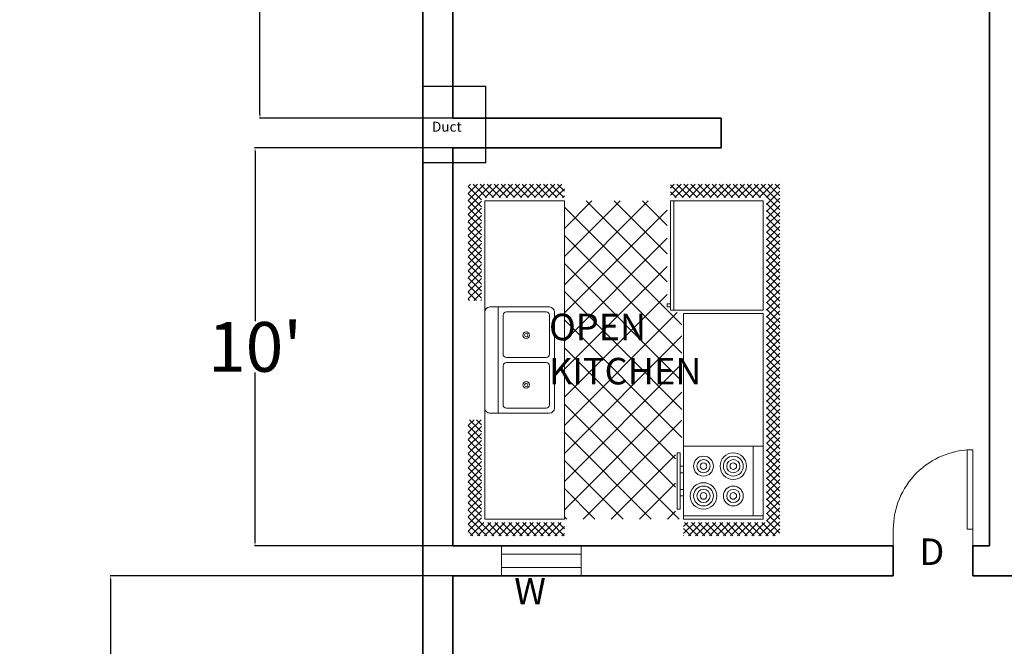
# Model space of a CAD drawing. Units: inches. Extents: x 371 to 1095, y -45 to 1219.
# Tile 8 of 18: x 371 to 668, y 421 to 610. Entities that reach past the tile are written whole.
import ezdxf

# ---------------------------------------------------------------- set-up
doc = ezdxf.new("R2010")
doc.units = ezdxf.units.IN
doc.header["$MEASUREMENT"] = 0
for name, color, linetype, lineweight in [('A-ANNO-DIMS', 2, 'Continuous', 18), ('A-ANNO-TEXT', 7, 'Continuous', 18), ('A-AREA-IDEN', 7, 'Continuous', 18), ('A-DOOR', 3, 'Continuous', 18), ('A-FLOR-FIXT', 9, 'Continuous', 18), ('A-FLOR-SHFT', 7, 'Continuous', 25), ('A-GLAZ', 4, 'Continuous', 18), ('A-WALL', 40, 'Continuous', 35), ('C-SITE-WALL', 40, 'Continuous', 35)]:
    doc.layers.add(name, color=color, linetype=linetype, lineweight=lineweight)
doc.styles.get("Standard").update_dxf_attribs({"font": 'arial.ttf'})
doc.dimstyles.get("Standard").update_dxf_attribs({"dimtxt": 1, "dimasz": 1, "dimexe": 0.18, "dimexo": 0.0625, "dimgap": 0.09, "dimtad": 0, "dimtih": 1, "dimtoh": 1, "dimdec": 0, "dimzin": 0, "dimdsep": 46, "dimlunit": 3, "dimtxsty": 'Standard', "dimcen": 0.09, "dimadec": 0, "dimazin": 0, "dimtfac": 1, "dimtdec": 0, "dimtofl": 0, "dimtmove": 0, "dimatfit": 3, "dimfxl": 1, "dimtolj": 1, "dimtzin": 0, "dimarcsym": 0})

# ---------------------------------------------------------------- blocks, each defined once
blk = doc.blocks.new('*U12')
for p, q in [((0, 0), (0, 5)), ((24, 0), (24, 5))]:
    blk.add_line(p, q)
blk.add_lwpolyline([(0, 0), (0, -24), (1.75, -24), (1.75, 0)], close=True)
blk.add_arc((0, 0), 24, 270, 0)
blk = doc.blocks.new('Kitchen Layout - 7 x 8 ft')
for p, q in [((-5, 81.32), (2.68, 89)), ((-5, 83.44), (0.56, 89)), ((-5, 85.56), (-1.56, 89)), ((-5, 87.68), (-3.68, 89)), ((-1, 84.97), (-5, 88.97)), ((-1, 82.85), (-5, 86.85)), ((1.09, 85), (-2.91, 89)), ((3.21, 85), (-0.79, 89)), ((0.81, 85), (4.81, 89)), ((5.34, 85), (1.34, 89)), ((2.93, 85), (6.93, 89)), ((7.46, 85), (3.46, 89)), ((5.05, 85), (9.05, 89)), ((9.58, 85), (5.58, 89)), ((7.17, 85), (11.17, 89)), ((11.7, 85), (7.7, 89)), ((9.29, 85), (13.29, 89)), ((13.82, 85), (9.82, 89)), ((11.41, 85), (15.41, 89)), ((15.94, 85), (11.94, 89)), ((13.53, 85), (17.53, 89)), ((18.06, 85), (14.06, 89)), ((15.65, 85), (19.65, 89)), ((20.18, 85), (16.18, 89)), ((17.78, 85), (21.78, 89)), ((22.31, 85), (18.31, 89)), ((19.9, 85), (23.9, 89)), ((24.43, 85), (20.43, 89)), ((22.02, 85), (26.02, 89)), ((26.55, 85), (22.55, 89)), ((24.14, 85), (28.14, 89)), ((28.67, 85), (24.67, 89)), ((26.26, 85), (30.26, 89)), ((30.79, 85), (26.79, 89)), ((28.38, 85), (32.38, 89)), ((32.91, 85), (28.91, 89)), ((30.5, 85), (34.5, 89)), ((35.03, 85), (31.03, 89)), ((32.63, 85), (36.63, 89)), ((37.16, 85), (33.16, 89)), ((34.75, 85), (38.75, 89)), ((39.28, 85), (35.28, 89)), ((36.87, 85), (40.87, 89)), ((41.4, 85), (37.4, 89)), ((38.99, 85), (42.99, 89)), ((43.52, 85), (39.52, 89)), ((41.11, 85), (45.11, 89)), ((45.64, 85), (41.64, 89)), ((43.23, 85), (47.23, 89)), ((47.76, 85), (43.76, 89)), ((45.35, 85), (49.35, 89)), ((49.88, 85), (45.88, 89)), ((47.47, 85), (51.47, 89)), ((52, 85), (48, 89)), ((49.6, 85), (53.6, 89)), ((54.13, 85), (50.13, 89)), ((51.72, 85), (55.72, 89)), ((56.25, 85), (52.25, 89)), ((53.84, 85), (57.84, 89)), ((58.37, 85), (54.37, 89)), ((55.96, 85), (59.96, 89)), ((60.49, 85), (56.49, 89)), ((58.08, 85), (62.08, 89)), ((62.61, 85), (58.61, 89)), ((60.2, 85), (64.2, 89)), ((64.73, 85), (60.73, 89)), ((62.32, 85), (66.32, 89)), ((66.85, 85), (62.85, 89)), ((64.45, 85), (68.45, 89)), ((68.97, 85), (64.97, 89)), ((66.57, 85), (70.57, 89)), ((71.1, 85), (67.1, 89)), ((68.69, 85), (72.69, 89)), ((73.22, 85), (69.22, 89)), ((70.81, 85), (74.81, 89)), ((75.34, 85), (71.34, 89)), ((72.93, 85), (76.93, 89)), ((77.46, 85), (73.46, 89)), ((75.05, 85), (79.05, 89)), ((79.58, 85), (75.58, 89)), ((77.17, 85), (81.17, 89)), ((81.7, 85), (77.7, 89)), ((79.29, 85), (83.29, 89)), ((83.82, 85), (79.82, 89)), ((81.42, 85), (85.42, 89)), ((85.95, 85), (81.95, 89)), ((83.54, 85), (87.54, 89)), ((88.07, 85), (84.07, 89)), ((85.66, 85), (89.66, 89)), ((90.19, 85), (86.19, 89)), ((87.78, 85), (91.78, 89)), ((92.31, 85), (88.31, 89)), ((89.9, 85), (93.9, 89)), ((94.43, 85), (90.43, 89)), ((92.02, 85), (96.02, 89)), ((96.55, 85), (92.55, 89)), ((94.14, 85), (98.14, 89)), ((101, 82.67), (94.67, 89)), ((96.27, 85), (100.27, 89)), ((101, 84.79), (96.79, 89)), ((97, 83.61), (101, 87.61)), ((101, 86.92), (98.92, 89)), ((-1, 80.73), (-5, 84.73)), ((34, 84), (96, 84)), ((34, 60), (34, 84)), ((96, 84), (96, 60)), ((97, 81.49), (101, 85.49)), ((101, 80.55), (97, 84.55)), ((97, 79.37), (101, 83.37)), ((-5, 79.19), (-1, 83.19)), ((-1, 78.61), (-5, 82.61)), ((-5, 77.07), (-1, 81.07)), ((-1, 76.49), (-5, 80.49)), ((74, 81), (95, 81)), ((101, 78.43), (97, 82.43)), ((97, 77.25), (101, 81.25)), ((101, 76.31), (97, 80.31)), ((-5, 74.95), (-1, 78.95)), ((-1, 74.36), (-5, 78.36)), ((97, 75.13), (101, 79.13)), ((101, 74.19), (97, 78.19)), ((-5, 72.83), (-1, 76.83)), ((-1, 72.24), (-5, 76.24)), ((-5, 70.71), (-1, 74.71)), ((97, 73.01), (101, 77.01)), ((101, 72.07), (97, 76.07)), ((97, 70.89), (101, 74.89)), ((-1, 70.12), (-5, 74.12)), ((-5, 68.59), (-1, 72.59)), ((-1, 68), (-5, 72)), ((101, 69.95), (97, 73.95)), ((97, 68.76), (101, 72.76)), ((101, 67.82), (97, 71.82)), ((-5, 66.47), (-1, 70.47)), ((-1, 65.88), (-5, 69.88)), ((97, 66.64), (101, 70.64)), ((101, 65.7), (97, 69.7)), ((97, 64.52), (101, 68.52)), ((-5, 64.35), (-1, 68.35)), ((-1, 63.76), (-5, 67.76)), ((-5, 62.22), (-1, 66.22)), ((-1, 61.64), (-5, 65.64)), ((101, 63.58), (97, 67.58)), ((97, 62.4), (101, 66.4)), ((101, 61.46), (97, 65.46)), ((-5, 60.1), (-1, 64.1)), ((-1, 59.52), (-5, 63.52)), ((97, 60.28), (101, 64.28)), ((100.34, 60), (97, 63.34)), ((-5, 57.98), (-1, 61.98)), ((-1, 57.39), (-5, 61.39)), ((-4.86, 56), (-1, 59.86)), ((10.4, 24), (45.9, 59.5)), ((18.88, 24), (54.38, 59.5)), ((27.37, 24), (62.87, 59.5)), ((33.03, 55.11), (37.41, 59.5)), ((96, 60), (34, 60)), ((35.85, 24), (71.35, 59.5)), ((76.2, 24), (40.7, 59.5)), ((84.68, 24), (49.18, 59.5)), ((93.17, 24), (57.67, 59.5)), ((96, 29.65), (66.15, 59.5)), ((80, 60), (80, 59)), ((82, 59), (82, 60)), ((87, 59), (87, 60)), ((89, 60), (89, 59)), ((98.22, 60), (97, 61.22)), ((98.84, 60), (101, 62.16)), ((100.96, 60), (101, 60.04)), ((-1.73, 56), (-5, 59.27)), ((-3.85, 56), (-5, 57.15)), ((-2.74, 56), (-1, 57.74)), ((0, 57), (33, 57)), ((67.71, 24), (33.68, 58.04)), ((44.34, 24), (77.84, 57.5)), ((52.82, 24), (86.32, 57.5)), ((61.31, 24), (96, 58.69)), ((96, 38.14), (76.64, 57.5)), ((96, 46.63), (85.13, 57.5)), ((96, 55.11), (93.57, 57.54)), ((0, 30.57), (24.43, 55)), ((0, 39.06), (15.94, 55)), ((0, 47.54), (7.46, 55)), ((1.91, 24), (32.91, 55)), ((33.77, 24), (2.77, 55)), ((42.26, 24), (11.26, 55)), ((50.74, 24), (19.74, 55)), ((59.23, 24), (28.23, 55)), ((31, 55), (31, 56)), ((32, 55), (31, 55)), ((32, 56), (32, 55)), ((25.29, 24), (0, 49.29)), ((69.79, 24), (96, 50.21)), ((78.28, 24), (96, 41.72)), ((16.8, 24), (0, 40.8)), ((86.76, 24), (96, 33.24)), ((8.32, 24), (0, 32.32)), ((-5, 21.92), (-2.92, 24)), ((-5, 19.8), (-1, 23.8)), ((-1, 21.33), (-3.67, 24)), ((-1, 23.45), (-1.55, 24)), ((0, 24), (96, 24)), ((0, 0), (0, 24)), ((95.25, 24), (96, 24.75)), ((96, 24), (96, 0)), ((97, 22.1), (98.9, 24)), ((97, 19.97), (101, 23.97)), ((101, 21.16), (98.16, 24)), ((101, 23.28), (100.28, 24)), ((-1, 19.21), (-5, 23.21)), ((-5, 17.68), (-1, 21.68)), ((-1, 17.09), (-5, 21.09)), ((101, 19.03), (97, 23.03)), ((97, 17.85), (101, 21.85)), ((101, 16.91), (97, 20.91)), ((-5, 15.55), (-1, 19.55)), ((-1, 14.97), (-5, 18.97)), ((47.25, 6.5), (47.25, 18.5)), ((48.75, 18.5), (48.75, 6.5)), ((97, 15.73), (101, 19.73)), ((101, 14.79), (97, 18.79)), ((-5, 13.43), (-1, 17.43)), ((-1, 12.85), (-5, 16.85)), ((-5, 11.31), (-1, 15.31)), ((97, 13.61), (101, 17.61)), ((101, 12.67), (97, 16.67)), ((97, 11.49), (101, 15.49)), ((-1, 10.73), (-5, 14.73)), ((-5, 9.19), (-1, 13.19)), ((-1, 8.6), (-5, 12.6)), ((101, 10.55), (97, 14.55)), ((97, 9.37), (101, 13.37)), ((101, 8.43), (97, 12.43)), ((-5, 7.07), (-1, 11.07)), ((-1, 6.48), (-5, 10.48)), ((-5, 4.95), (-1, 8.95)), ((97, 7.25), (101, 11.25)), ((101, 6.31), (97, 10.31)), ((97, 5.12), (101, 9.12)), ((-1, 4.36), (-5, 8.36)), ((-5, 2.83), (-1, 6.83)), ((-1, 2.24), (-5, 6.24)), ((101, 4.18), (97, 8.18)), ((97, 3), (101, 7)), ((101, 2.06), (97, 6.06)), ((-5, 0.71), (-1, 4.71)), ((-1, 0.12), (-5, 4.12)), ((64, 4), (32, 4)), ((97, 0.88), (101, 4.88)), ((101, -0.06), (97, 3.94)), ((-5, -1.42), (-1, 2.58)), ((2, -5), (-5, 2)), ((-5, -3.54), (-1, 0.46)), ((96, 0), (0, 0)), ((93.24, -5), (101, 2.76)), ((95.36, -5), (101, 0.64)), ((101, -2.18), (97, 1.82)), ((-0.12, -5), (-5, -0.12)), ((-2.25, -5), (-5, -2.25)), ((-4.34, -5), (-0.34, -1)), ((-2.22, -5), (1.78, -1)), ((-0.1, -5), (3.9, -1)), ((4.12, -5), (0.12, -1)), ((2.02, -5), (6.02, -1)), ((6.24, -5), (2.24, -1)), ((4.14, -5), (8.14, -1)), ((8.36, -5), (4.36, -1)), ((6.27, -5), (10.27, -1)), ((10.48, -5), (6.48, -1)), ((8.39, -5), (12.39, -1)), ((12.6, -5), (8.6, -1)), ((10.51, -5), (14.51, -1)), ((14.73, -5), (10.73, -1)), ((12.63, -5), (16.63, -1)), ((16.85, -5), (12.85, -1)), ((14.75, -5), (18.75, -1)), ((18.97, -5), (14.97, -1)), ((16.87, -5), (20.87, -1)), ((21.09, -5), (17.09, -1)), ((18.99, -5), (22.99, -1)), ((23.21, -5), (19.21, -1)), ((21.11, -5), (25.11, -1)), ((25.33, -5), (21.33, -1)), ((23.24, -5), (27.24, -1)), ((27.45, -5), (23.45, -1)), ((25.36, -5), (29.36, -1)), ((29.57, -5), (25.57, -1)), ((27.48, -5), (30, -2.48)), ((30, -3.3), (27.7, -1)), ((30, -1.18), (29.82, -1)), ((66, -2.54), (67.54, -1)), ((66, -4.66), (69.66, -1)), ((69.88, -5), (66, -1.12)), ((67.78, -5), (71.78, -1)), ((72, -5), (68, -1)), ((69.9, -5), (73.9, -1)), ((74.12, -5), (70.12, -1)), ((72.03, -5), (76.03, -1)), ((76.24, -5), (72.24, -1)), ((74.15, -5), (78.15, -1)), ((78.36, -5), (74.36, -1)), ((76.27, -5), (80.27, -1)), ((80.49, -5), (76.49, -1)), ((78.39, -5), (82.39, -1)), ((82.61, -5), (78.61, -1)), ((80.51, -5), (84.51, -1)), ((84.73, -5), (80.73, -1)), ((82.63, -5), (86.63, -1)), ((86.85, -5), (82.85, -1)), ((84.75, -5), (88.75, -1)), ((88.97, -5), (84.97, -1)), ((86.88, -5), (90.88, -1)), ((91.09, -5), (87.09, -1)), ((89, -5), (93, -1)), ((93.21, -5), (89.21, -1)), ((91.12, -5), (95.12, -1)), ((95.34, -5), (91.34, -1)), ((97.46, -5), (93.46, -1)), ((99.58, -5), (95.58, -1)), ((101, -4.3), (97, -0.3)), ((97.48, -5), (101, -1.48)), ((-4.37, -5), (-5, -4.37)), ((29.6, -5), (30, -4.6)), ((67.76, -5), (66, -3.24)), ((99.6, -5), (101, -3.6))]:
    blk.add_line(p, q)
for points in [[(0, 56), (0, 84), (33, 84), (33, 56)], [(74, 60), (74, 84), (95, 84), (95, 60)], [(76, 58), (76, 59), (93, 59), (93, 58)]]:
    blk.add_lwpolyline(points, close=True)
for points in [[(33.5, 21), (62.5, 21)], [(32, 1.5), (32, 19.5)], [(33.5, 6.5), (33.5, 18.5)], [(34.5, 19.5), (46.25, 19.5)], [(49.75, 19.5), (61.5, 19.5)], [(62.5, 18.5), (62.5, 6.5)], [(64, 19.5), (64, 1.5)], [(46.25, 5.5), (34.5, 5.5)], [(61.5, 5.5), (49.75, 5.5)], [(62.5, 0), (33.5, 0)]]:
    blk.add_lwpolyline(points)
for centre, radius in [((80, 75), 4), ((80, 75), 3), ((89, 75), 3), ((80, 75), 2), ((80, 75), 1), ((89, 75), 2), ((89, 75), 1), ((80, 66), 3), ((89, 66), 4), ((89, 66), 3), ((80, 66), 2), ((80, 66), 1), ((89, 66), 2), ((89, 66), 1), ((40.5, 12.5), 1), ((40.5, 12.5), 0.5), ((55.5, 12.5), 1), ((55.5, 12.5), 0.5)]:
    blk.add_circle(centre, radius)
for centre, radius, start, end in [((33.5, 19.5), 1.5, 90, 180), ((62.5, 19.5), 1.5, 0, 90), ((34.5, 18.5), 1, 90, 180), ((46.25, 18.5), 1, 0, 90), ((49.75, 18.5), 1, 90, 180), ((61.5, 18.5), 1, 0, 90), ((34.5, 6.5), 1, 180, 270), ((46.25, 6.5), 1, 270, 0), ((49.75, 6.5), 1, 180, 270), ((61.5, 6.5), 1, 270, 0), ((33.5, 1.5), 1.5, 180, 270), ((62.5, 1.5), 1.5, 270, 0)]:
    blk.add_arc(centre, radius, start, end)
blk = doc.blocks.new('*D20')
at = {"layer": 'A-ANNO-DIMS', "color": 0, "lineweight": -2, "transparency": 16777216}
for p, q in [((501.75, 796.03), (443.44, 796.03)), ((443.62, 795.03), (443.62, 695.77)), ((443.62, 581.03), (443.62, 680.28)), ((501.75, 580.03), (443.44, 580.03))]:
    blk.add_line(p, q, dxfattribs=at)
at = {"layer": 'A-ANNO-DIMS', "color": 0, "transparency": 16777216}
for points in [[(443.46, 795.03), (443.79, 795.03), (443.62, 796.03)], [(443.46, 581.03), (443.79, 581.03), (443.62, 580.03)]]:
    blk.add_solid(points, dxfattribs=at)
at = {"layer": 'Defpoints', "color": 0, "transparency": 16777216}
for p in [(501.81, 796.03), (443.62, 580.03), (501.81, 580.03)]:
    blk.add_point(p, dxfattribs=at)
at = {"layer": 'A-ANNO-DIMS', "color": 0, "transparency": 16777216, "insert": (443.62, 688.03), "char_height": 1, "attachment_point": 5}
blk.add_mtext("\\A1;{\\H15x;18'}", dxfattribs=at)
blk = doc.blocks.new('*D21')
at = {"layer": 'A-ANNO-DIMS', "color": 0, "lineweight": -2, "transparency": 16777216}
for p, q in [((501.75, 571.03), (441.97, 571.03)), ((442.15, 570.03), (442.15, 518.77)), ((442.15, 452.03), (442.15, 503.28)), ((501.75, 451.03), (441.97, 451.03))]:
    blk.add_line(p, q, dxfattribs=at)
at = {"layer": 'A-ANNO-DIMS', "color": 0, "transparency": 16777216}
for points in [[(441.98, 570.03), (442.31, 570.03), (442.15, 571.03)], [(441.98, 452.03), (442.31, 452.03), (442.15, 451.03)]]:
    blk.add_solid(points, dxfattribs=at)
at = {"layer": 'Defpoints', "color": 0, "transparency": 16777216}
for p in [(501.81, 571.03), (442.15, 451.03), (501.81, 451.03)]:
    blk.add_point(p, dxfattribs=at)
at = {"layer": 'A-ANNO-DIMS', "color": 0, "transparency": 16777216, "insert": (442.15, 511.03), "char_height": 1, "attachment_point": 5}
blk.add_mtext("\\A1;{\\H15x;10'}", dxfattribs=at)
blk = doc.blocks.new('*D25')
at = {"layer": 'A-ANNO-DIMS', "color": 0, "lineweight": -2, "transparency": 16777216}
for p, q in [((501.75, 442.03), (398.38, 442.03)), ((398.56, 441.03), (398.56, 274.28)), ((398.56, 92.03), (398.56, 258.77)), ((501.75, 91.03), (398.38, 91.03))]:
    blk.add_line(p, q, dxfattribs=at)
at = {"layer": 'A-ANNO-DIMS', "color": 0, "transparency": 16777216}
for points in [[(398.4, 441.03), (398.73, 441.03), (398.56, 442.03)], [(398.4, 92.03), (398.73, 92.03), (398.56, 91.03)]]:
    blk.add_solid(points, dxfattribs=at)
at = {"layer": 'Defpoints', "color": 0, "transparency": 16777216}
for p in [(501.81, 442.03), (398.56, 91.03), (501.81, 91.03)]:
    blk.add_point(p, dxfattribs=at)
at = {"layer": 'A-ANNO-DIMS', "color": 0, "transparency": 16777216, "insert": (398.56, 266.53), "char_height": 1, "attachment_point": 5}
blk.add_mtext('\\A1;{\\H15x;29\'-3"}', dxfattribs=at)
blk = doc.blocks.new('SHAFT-KITCHEN')
for p, q in [((19, 23), (0, 23)), ((0, 23), (0, 0)), ((19, 0), (19, 23)), ((19, 0), (0, 0))]:
    blk.add_line(p, q)

msp = doc.modelspace()

# ---------------------------------------------------------------- linework, layer by layer
at = {"layer": 'A-GLAZ'}
for p, q in [((516.54, 448.5), (540.54, 448.5)), ((516.54, 444.5), (540.54, 444.5))]:
    msp.add_line(p, q, dxfattribs=at)
msp.add_lwpolyline([(516.54, 442.03), (540.54, 442.03), (540.54, 451.03), (516.54, 451.03)], close=True, dxfattribs=at)
at = {"layer": 'A-WALL'}
for p, q in [((492.81, 982.03), (492.81, 82.03)), ((501.81, 796.03), (501.81, 580.03)), ((663.81, 796.03), (663.81, 451.03)), ((501.81, 580.03), (582.81, 580.03)), ((582.81, 580.03), (582.81, 571.03)), ((501.81, 571.03), (582.81, 571.03)), ((501.81, 571.03), (501.81, 451.03)), ((501.81, 451.03), (634.81, 451.03)), ((634.81, 451.03), (634.81, 442.03)), ((658.81, 442.03), (658.81, 451.03)), ((658.81, 451.03), (663.81, 451.03)), ((501.81, 442.03), (634.81, 442.03)), ((658.81, 442.03), (663.81, 442.03)), ((663.81, 442.03), (677.81, 442.03))]:
    msp.add_line(p, q, dxfattribs=at)
at = {"layer": 'C-SITE-WALL'}
msp.add_line((501.81, 442.03), (501.81, 91.03), dxfattribs=at)

# ---------------------------------------------------------------- block references
at = {"layer": 'A-DOOR', "rotation": 180}
msp.add_blockref('*U12', (658.81, 456.03), dxfattribs=at)
at = {"layer": 'A-FLOR-FIXT', "rotation": 270}
msp.add_blockref('Kitchen Layout - 7 x 8 ft', (511.51, 555.07), dxfattribs=at)
at = {"layer": 'A-FLOR-SHFT'}
msp.add_blockref('SHAFT-KITCHEN', (492.81, 566.58), dxfattribs=at)

# ---------------------------------------------------------------- texts
at = {"layer": 'A-ANNO-TEXT', "char_height": 8, "attachment_point": 1}
for s, insert in [('D', (642.7, 453.25)), ('W', (520.36, 441.37))]:
    msp.add_mtext_dynamic_manual_height_columns(s, width=17.4938, gutter_width=1, heights=[0], dxfattribs=dict(at, insert=insert))
at = {"layer": 'A-AREA-IDEN', "attachment_point": 1}
for s, width, insert, char_height in [('Duct', 31.9108, (495.56, 578.95), 3), ('OPEN KITCHEN ', 53.6318, (530.87, 521.05), 8)]:
    msp.add_mtext_dynamic_manual_height_columns(s, width=width, gutter_width=1, heights=[0], dxfattribs=dict(at, insert=insert, char_height=char_height))

# ---------------------------------------------------------------- dimensions: what is measured, and where the dimension line sits
at = {"layer": 'A-ANNO-DIMS'}
for base, p1, p2, picture, middle in [((443.62, 580.03), (501.81, 796.03), (501.81, 580.03), '*D20', (443.62, 688.03)), ((442.15, 451.03), (501.81, 571.03), (501.81, 451.03), '*D21', (442.15, 511.03)), ((398.56, 91.03), (501.81, 442.03), (501.81, 91.03), '*D25', (398.56, 266.53))]:
    dim = msp.add_linear_dim(base=base, p1=p1, p2=p2, angle=90, text='{\\H15x;<>}', dimstyle='Standard', override={"dimclrd": 0, "dimclre": 0, "dimclrt": 0}, dxfattribs=at)
    dim.commit()
    dim.dimension.update_dxf_attribs({"geometry": picture, "text_midpoint": middle})

doc.saveas('drawing.dxf')
